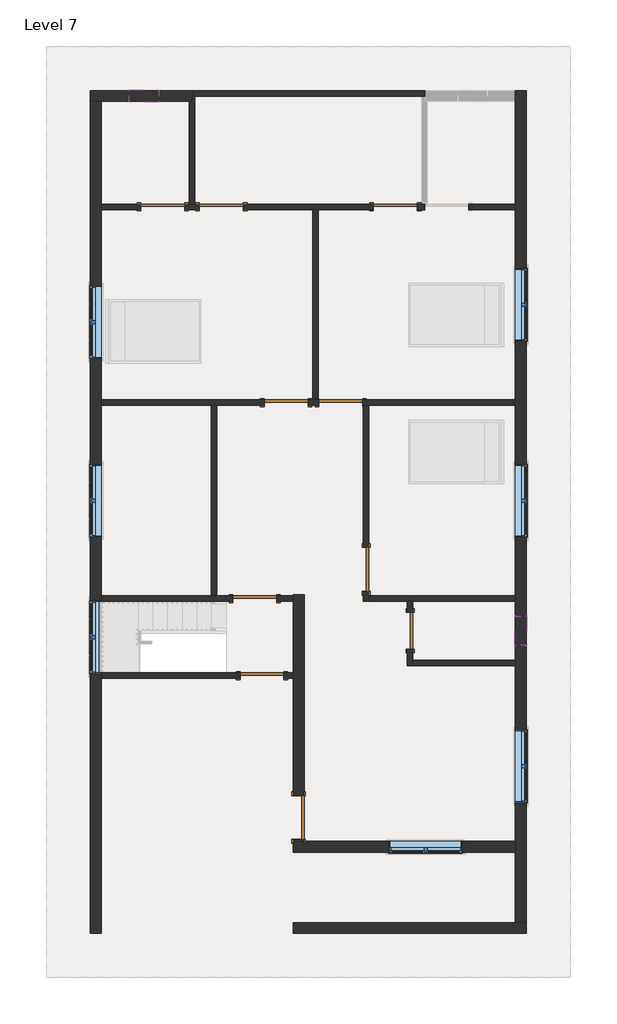
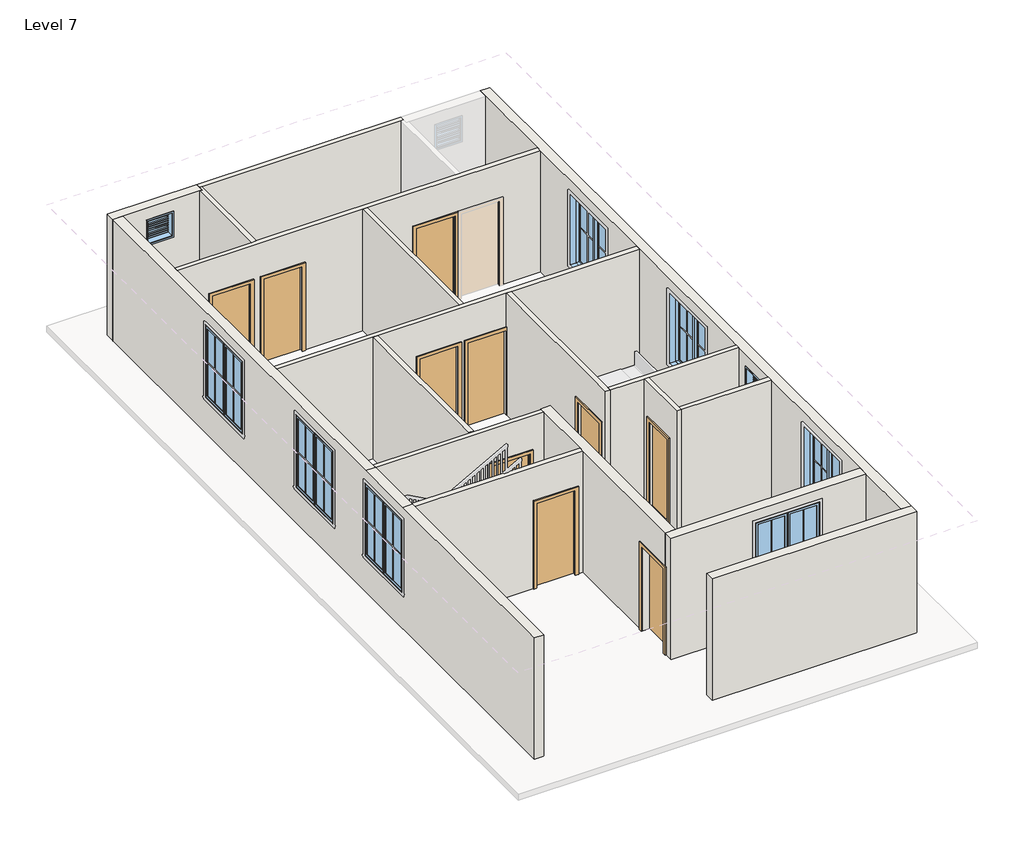
# One storey, part 1 of 3: 18 walls, 10 doors, 9 windows.
"""IFC4 building model written with IfcOpenShell, lengths in millimetres."""

from ifc_helpers import new_model, si_unit, frame, origin, place, context, project, spatial, polyline, outline, extrude, faceted_brep, transform, mapped, element, save
from components import door_78caadf7, single_flush_door_3_e5f9f3c4, single_flush_door_3_305aa2a5, single_flush_door_3_0ca8825f, window_casement_double_win_5_f93960c7, window_f2d8fef0

model = new_model("IFC4")

# Units and contexts
model_context = context("Model", 3, world=origin())
ifc_project = project(units=[si_unit("LENGTHUNIT", "METRE", prefix="MILLI")], contexts=[model_context])

# Site, building, storey
site = spatial("IfcSite", under=ifc_project)
building = spatial("IfcBuilding", under=site)
storey = spatial("IfcBuildingStorey", under=building, Name="Level 7", Elevation=16002.0)

# Doors
placement = place(None, origin())
door_shape = door_78caadf7(model_context)
element("IfcDoor", 1, ObjectType="Single-Flush : DOOR 2'6\"", at=placement, inside=storey, context=model_context, shape_type="MappedRepresentation", body=[
    mapped(door_shape, transform((860.2379845, -2779.6065691, 16002.0), x_axis=(0.0, 1.0, 0.0), y_axis=(-1.0, 0.0, 0.0), z_axis=(0.0, 0.0, 1.0))),
])
single_flush_door_3_shape = single_flush_door_3_e5f9f3c4(model_context)
element("IfcDoor", 2, ObjectType="Single-Flush : DOOR 3'", at=placement, inside=storey, context=model_context, shape_type="MappedRepresentation", body=[
    mapped(single_flush_door_3_shape, transform((-54.1620155, -1503.2565691, 16002.0), x_axis=(0.0, -1.0, 0.0), y_axis=(1.0, 0.0, 0.0), z_axis=(0.0, 0.0, 1.0))),
])
element("IfcDoor", 3, ObjectType="Single-Flush : DOOR 3'", at=placement, inside=storey, context=model_context, shape_type="MappedRepresentation", body=[
    mapped(single_flush_door_3_shape, transform((-1717.8620155, 1963.8434309, 16002.0), x_axis=(1.0, 0.0, 0.0), y_axis=(0.0, 1.0, 0.0), z_axis=(0.0, 0.0, 1.0))),
])
element("IfcDoor", 4, ObjectType="Single-Flush : DOOR 3'", at=placement, inside=storey, context=model_context, shape_type="MappedRepresentation", body=[
    mapped(single_flush_door_3_shape, transform((-2371.9120155, -2112.8565691, 16002.0), x_axis=(1.0, 0.0, 0.0), y_axis=(0.0, 1.0, 0.0), z_axis=(0.0, 0.0, 1.0))),
])
element("IfcDoor", 5, ObjectType="Single-Flush : DOOR 3'", at=placement, inside=storey, context=model_context, shape_type="MappedRepresentation", body=[
    mapped(single_flush_door_3_shape, transform((-2219.5120155, -3713.0565691, 16002.0), x_axis=(1.0, 0.0, 0.0), y_axis=(0.0, 1.0, 0.0), z_axis=(0.0, 0.0, 1.0))),
])
element("IfcDoor", 6, ObjectType="Single-Flush : DOOR 3'", at=placement, inside=storey, context=model_context, shape_type="MappedRepresentation", body=[
    mapped(single_flush_door_3_shape, transform((-4283.2620155, 6040.5434309, 16002.0), x_axis=(1.0, 0.0, 0.0), y_axis=(0.0, 1.0, 0.0), z_axis=(0.0, 0.0, 1.0))),
])
element("IfcDoor", 7, ObjectType="Single-Flush : DOOR 3'", at=placement, inside=storey, context=model_context, shape_type="MappedRepresentation", body=[
    mapped(single_flush_door_3_shape, transform((555.4379845, 6040.5434309, 16002.0), x_axis=(1.0, 0.0, 0.0), y_axis=(0.0, 1.0, 0.0), z_axis=(0.0, 0.0, 1.0))),
])
single_flush_door_3_2_shape = single_flush_door_3_305aa2a5(model_context)
element("IfcDoor", 8, ObjectType="Single-Flush : DOOR 3'", at=placement, inside=storey, context=model_context, shape_type="MappedRepresentation", body=[
    mapped(single_flush_door_3_2_shape, transform((-581.2120155, 1963.8434309, 16002.0), x_axis=(-1.0, 0.0, 0.0), y_axis=(0.0, -1.0, 0.0), z_axis=(0.0, 0.0, 1.0))),
])
element("IfcDoor", 9, ObjectType="Single-Flush : DOOR 3'", at=placement, inside=storey, context=model_context, shape_type="MappedRepresentation", body=[
    mapped(single_flush_door_3_2_shape, transform((-3064.0620155, 6040.5434309, 16002.0), x_axis=(-1.0, 0.0, 0.0), y_axis=(0.0, -1.0, 0.0), z_axis=(0.0, 0.0, 1.0))),
])
single_flush_door_3_3_shape = single_flush_door_3_0ca8825f(model_context)
element("IfcDoor", 10, ObjectType="Single-Flush : DOOR 3'", at=placement, inside=storey, context=model_context, shape_type="MappedRepresentation", body=[
    mapped(single_flush_door_3_3_shape, transform((-1457.5120155, -6665.8065691, 16002.0), x_axis=(0.0, -1.0, 0.0), y_axis=(1.0, 0.0, 0.0), z_axis=(0.0, 0.0, 1.0))),
])

# Walls
element("IfcWall", 11, ObjectType="WALL 4.5\"", at=placement, inside=storey, context=model_context, shape_type="Brep", body=[
    faceted_brep([(-3673.6620155, 8345.5934309, 16002.0), (-3616.5120155, 8345.5934309, 16002.0), (1107.8879845, 8345.5934309, 16002.0), (1165.0379845, 8345.5934309, 16002.0), (1165.0379845, 8345.5934309, 19050.0), (1107.8879845, 8345.5934309, 19050.0), (-3616.5120155, 8345.5934309, 19050.0), (-3673.6620155, 8345.5934309, 19050.0), (-3673.6620155, 8459.8934309, 16002.0), (-3673.6620155, 8459.8934309, 19050.0), (1165.0379845, 8459.8934309, 19050.0), (1165.0379845, 8459.8934309, 16002.0)], [[[0, 1, 2, 3, 4, 5, 6, 7]], [[8, 9, 10, 11]], [[3, 2, 1, 0, 8, 11]], [[4, 3, 11, 10]], [[0, 7, 9, 8]], [[7, 6, 5, 4, 10, 9]]]),
])
element("IfcWall", 12, ObjectType="WALL 4.5\"", at=placement, inside=storey, context=model_context, shape_type="SweptSolid", body=[
    extrude(outline(polyline([(-3730.8120155, 6097.6934309), (-3730.8120155, 8231.2934309), (-3673.6620155, 8231.2934309), (-3673.6620155, 8345.5934309), (-3616.5120155, 8345.5934309), (-3616.5120155, 6097.6934309), (-3730.8120155, 6097.6934309)])), frame((0.0, 0.0, 16002.0), z_axis=(0.0, 0.0, 1.0), x_axis=(1.0, 0.0, 0.0)), (0.0, 0.0, 1.0), 3048.0),
])
element("IfcWall", 13, ObjectType="WALL 4.5\"", at=placement, inside=storey, context=model_context, shape_type="Brep", body=[
    faceted_brep([(1165.0379845, 6097.6934309, 18135.6), (1165.0379845, 6097.6934309, 16002.0), (1107.8879845, 6097.6934309, 16002.0), (1012.6379845, 6097.6934309, 16002.0), (1012.6379845, 6097.6934309, 18135.6), (98.2379845, 6097.6934309, 18135.6), (98.2379845, 6097.6934309, 16002.0), (-2606.8620155, 6097.6934309, 16002.0), (-2606.8620155, 6097.6934309, 18135.6), (-3521.2620155, 6097.6934309, 18135.6), (-3521.2620155, 6097.6934309, 16002.0), (-3616.5120155, 6097.6934309, 16002.0), (-3730.8120155, 6097.6934309, 16002.0), (-3826.0620155, 6097.6934309, 16002.0), (-3826.0620155, 6097.6934309, 18135.6), (-4740.4620155, 6097.6934309, 18135.6), (-4740.4620155, 6097.6934309, 16002.0), (-5559.6120155, 6097.6934309, 16002.0), (-5559.6120155, 6097.6934309, 19050.0), (-3730.8120155, 6097.6934309, 19050.0), (-3616.5120155, 6097.6934309, 19050.0), (1107.8879845, 6097.6934309, 19050.0), (1222.1879845, 6097.6934309, 19050.0), (3050.9879845, 6097.6934309, 19050.0), (3050.9879845, 6097.6934309, 16002.0), (2079.4379845, 6097.6934309, 16002.0), (2079.4379845, 6097.6934309, 18135.6), (1012.6379845, 5983.3934309, 16002.0), (1165.0379845, 5983.3934309, 16002.0), (1165.0379845, 5983.3934309, 18135.6), (2079.4379845, 5983.3934309, 18135.6), (2079.4379845, 5983.3934309, 16002.0), (3050.9879845, 5983.3934309, 16002.0), (3050.9879845, 5983.3934309, 19050.0), (-1051.1120155, 5983.3934309, 19050.0), (-1165.4120155, 5983.3934309, 19050.0), (-5559.6120155, 5983.3934309, 19050.0), (-5559.6120155, 5983.3934309, 16002.0), (-4740.4620155, 5983.3934309, 16002.0), (-4740.4620155, 5983.3934309, 18135.6), (-3826.0620155, 5983.3934309, 18135.6), (-3826.0620155, 5983.3934309, 16002.0), (-3521.2620155, 5983.3934309, 16002.0), (-3521.2620155, 5983.3934309, 18135.6), (-2606.8620155, 5983.3934309, 18135.6), (-2606.8620155, 5983.3934309, 16002.0), (-1165.4120155, 5983.3934309, 16002.0), (-1051.1120155, 5983.3934309, 16002.0), (98.2379845, 5983.3934309, 16002.0), (98.2379845, 5983.3934309, 18135.6), (1012.6379845, 5983.3934309, 18135.6)], [[[0, 1, 2, 3, 4, 5, 6, 7, 8, 9, 10, 11, 12, 13, 14, 15, 16, 17, 18, 19, 20, 21, 22, 23, 24, 25, 26]], [[27, 28, 29, 30, 31, 32, 33, 34, 35, 36, 37, 38, 39, 40, 41, 42, 43, 44, 45, 46, 47, 48, 49, 50]], [[38, 37, 17, 16]], [[13, 12, 11, 10, 42, 41]], [[48, 47, 46, 45, 7, 6]], [[25, 24, 32, 31]], [[3, 2, 1, 28, 27]], [[18, 17, 37, 36]], [[24, 23, 33, 32]], [[14, 13, 41, 40]], [[15, 14, 40, 39]], [[16, 15, 39, 38]], [[43, 42, 10, 9]], [[44, 43, 9, 8]], [[45, 44, 8, 7]], [[4, 3, 27, 50]], [[5, 4, 50, 49]], [[6, 5, 49, 48]], [[29, 28, 1, 0]], [[30, 29, 0, 26]], [[31, 30, 26, 25]], [[23, 22, 21, 20, 19, 18, 36, 35, 34, 33]]]),
])
element("IfcWall", 14, ObjectType="WALL 4.5\"", at=placement, inside=storey, context=model_context, shape_type="SweptSolid", body=[
    extrude(outline(polyline([(-1165.4120155, 2020.9934309), (-1165.4120155, 5983.3934309), (-1051.1120155, 5983.3934309), (-1051.1120155, 2020.9934309), (-1165.4120155, 2020.9934309)])), frame((0.0, 0.0, 16002.0), z_axis=(0.0, 0.0, 1.0), x_axis=(1.0, 0.0, 0.0)), (0.0, 0.0, 1.0), 3048.0),
])
element("IfcWall", 15, ObjectType="WALL 4.5\"", at=placement, inside=storey, context=model_context, shape_type="Brep", body=[
    faceted_brep([(-1260.6620155, 1906.6934309, 18135.6), (-1260.6620155, 1906.6934309, 16002.0), (-1038.4120155, 1906.6934309, 16002.0), (-1038.4120155, 1906.6934309, 18135.6), (-124.0120155, 1906.6934309, 18135.6), (-124.0120155, 1906.6934309, 16002.0), (-111.3120155, 1906.6934309, 16002.0), (2.9879845, 1906.6934309, 16002.0), (3050.9879845, 1906.6934309, 16002.0), (3050.9879845, 1906.6934309, 19050.0), (2.9879845, 1906.6934309, 19050.0), (-111.3120155, 1906.6934309, 19050.0), (-3159.3120155, 1906.6934309, 19050.0), (-3273.6120155, 1906.6934309, 19050.0), (-5559.6120155, 1906.6934309, 19050.0), (-5559.6120155, 1906.6934309, 16002.0), (-3273.6120155, 1906.6934309, 16002.0), (-3159.3120155, 1906.6934309, 16002.0), (-2175.0620155, 1906.6934309, 16002.0), (-2175.0620155, 1906.6934309, 18135.6), (-1038.4120155, 2020.9934309, 16002.0), (-1051.1120155, 2020.9934309, 16002.0), (-1165.4120155, 2020.9934309, 16002.0), (-1260.6620155, 2020.9934309, 16002.0), (-1260.6620155, 2020.9934309, 18135.6), (-2175.0620155, 2020.9934309, 18135.6), (-2175.0620155, 2020.9934309, 16002.0), (-5559.6120155, 2020.9934309, 16002.0), (-5559.6120155, 2020.9934309, 19050.0), (-1165.4120155, 2020.9934309, 19050.0), (-1051.1120155, 2020.9934309, 19050.0), (3050.9879845, 2020.9934309, 19050.0), (3050.9879845, 2020.9934309, 16002.0), (-124.0120155, 2020.9934309, 16002.0), (-124.0120155, 2020.9934309, 18135.6), (-1038.4120155, 2020.9934309, 18135.6)], [[[0, 1, 2, 3, 4, 5, 6, 7, 8, 9, 10, 11, 12, 13, 14, 15, 16, 17, 18, 19]], [[20, 21, 22, 23, 24, 25, 26, 27, 28, 29, 30, 31, 32, 33, 34, 35]], [[33, 32, 8, 7, 6, 5]], [[2, 1, 23, 22, 21, 20]], [[18, 17, 16, 15, 27, 26]], [[15, 14, 28, 27]], [[9, 8, 32, 31]], [[3, 2, 20, 35]], [[4, 3, 35, 34]], [[5, 4, 34, 33]], [[24, 23, 1, 0]], [[25, 24, 0, 19]], [[26, 25, 19, 18]], [[14, 13, 12, 11, 10, 9, 31, 30, 29, 28]]]),
])
element("IfcWall", 16, ObjectType="WALL 4.5\"", at=placement, inside=storey, context=model_context, shape_type="SweptSolid", body=[
    extrude(outline(polyline([(-3273.6120155, -2032.8465691), (-3273.6120155, 1906.6934309), (-3159.3120155, 1906.6934309), (-3159.3120155, -2032.8465691), (-3273.6120155, -2032.8465691)])), frame((0.0, 0.0, 16002.0), z_axis=(0.0, 0.0, 1.0), x_axis=(1.0, 0.0, 0.0)), (0.0, 0.0, 1.0), 3048.0),
])
element("IfcWall", 17, ObjectType="WALL 4.5\"", at=placement, inside=storey, context=model_context, shape_type="SweptSolid", body=[
    extrude(outline(polyline([(18135.6, -1914.7120155), (16002.0, -1914.7120155), (16002.0, -1571.8120155), (19050.0, -1571.8120155), (19050.0, -5559.6120155), (16002.0, -5559.6120155), (16002.0, -2829.1120155), (18135.6, -2829.1120155), (18135.6, -1914.7120155)])), frame((0.0, -2170.0065691, 0.0), z_axis=(0.0, 1.0, 0.0), x_axis=(0.0, 0.0, 1.0)), (0.0, 0.0, 1.0), 114.3),
])
element("IfcWall", 18, ObjectType="WALL 4.5\"", at=placement, inside=storey, context=model_context, shape_type="SweptSolid", body=[
    extrude(outline(polyline([(18135.6, -1762.3120155), (16002.0, -1762.3120155), (16002.0, -1571.8120155), (19050.0, -1571.8120155), (19050.0, -5559.6120155), (16002.0, -5559.6120155), (16002.0, -2676.7120155), (18135.6, -2676.7120155), (18135.6, -1762.3120155)])), frame((0.0, -3770.2065691, 0.0), z_axis=(0.0, 1.0, 0.0), x_axis=(0.0, 0.0, 1.0)), (0.0, 0.0, 1.0), 114.3),
])
element("IfcWall", 19, ObjectType="WALL 4.5\"", at=placement, inside=storey, context=model_context, shape_type="Brep", body=[
    faceted_brep([(-111.3120155, -1960.4565691, 18135.6), (-111.3120155, -1960.4565691, 16002.0), (-111.3120155, -2170.0065691, 16002.0), (-111.3120155, -2170.0065691, 19050.0), (-111.3120155, 1906.6934309, 19050.0), (-111.3120155, 1906.6934309, 16002.0), (-111.3120155, -1046.0565691, 16002.0), (-111.3120155, -1046.0565691, 18135.6), (2.9879845, -2170.0065691, 16002.0), (2.9879845, -2055.7065691, 16002.0), (2.9879845, -1960.4565691, 16002.0), (2.9879845, -1960.4565691, 18135.6), (2.9879845, -1046.0565691, 18135.6), (2.9879845, -1046.0565691, 16002.0), (2.9879845, 1906.6934309, 16002.0), (2.9879845, 1906.6934309, 19050.0), (2.9879845, -2055.7065691, 19050.0), (2.9879845, -2170.0065691, 19050.0)], [[[0, 1, 2, 3, 4, 5, 6, 7]], [[8, 9, 10, 11, 12, 13, 14, 15, 16, 17]], [[6, 5, 14, 13]], [[2, 1, 10, 9, 8]], [[5, 4, 15, 14]], [[3, 2, 8, 17]], [[11, 10, 1, 0]], [[12, 11, 0, 7]], [[13, 12, 7, 6]], [[4, 3, 17, 16, 15]]]),
])
element("IfcWall", 20, ObjectType="WALL 4.5\"", at=placement, inside=storey, context=model_context, shape_type="Brep", body=[
    faceted_brep([(2.9879845, -2170.0065691, 16002.0), (803.0879845, -2170.0065691, 16002.0), (917.3879845, -2170.0065691, 16002.0), (3050.9879845, -2170.0065691, 16002.0), (3050.9879845, -2170.0065691, 19050.0), (917.3879845, -2170.0065691, 19050.0), (803.0879845, -2170.0065691, 19050.0), (2.9879845, -2170.0065691, 19050.0), (2.9879845, -2055.7065691, 16002.0), (2.9879845, -2055.7065691, 19050.0), (3050.9879845, -2055.7065691, 19050.0), (3050.9879845, -2055.7065691, 16002.0)], [[[0, 1, 2, 3, 4, 5, 6, 7]], [[8, 9, 10, 11]], [[3, 2, 1, 0, 8, 11]], [[0, 7, 9, 8]], [[4, 3, 11, 10]], [[7, 6, 5, 4, 10, 9]]]),
])
element("IfcWall", 21, ObjectType="WALL 4.5\"", at=placement, inside=storey, context=model_context, shape_type="Brep", body=[
    faceted_brep([(803.0879845, -2170.0065691, 16002.0), (803.0879845, -2398.6065691, 16002.0), (803.0879845, -2398.6065691, 18135.6), (803.0879845, -3160.6065691, 18135.6), (803.0879845, -3160.6065691, 16002.0), (803.0879845, -3503.5065691, 16002.0), (803.0879845, -3503.5065691, 19050.0), (803.0879845, -2170.0065691, 19050.0), (917.3879845, -2398.6065691, 18135.6), (917.3879845, -2398.6065691, 16002.0), (917.3879845, -2170.0065691, 16002.0), (917.3879845, -2170.0065691, 19050.0), (917.3879845, -3389.2065691, 19050.0), (917.3879845, -3503.5065691, 19050.0), (917.3879845, -3503.5065691, 16002.0), (917.3879845, -3389.2065691, 16002.0), (917.3879845, -3160.6065691, 16002.0), (917.3879845, -3160.6065691, 18135.6)], [[[0, 1, 2, 3, 4, 5, 6, 7]], [[8, 9, 10, 11, 12, 13, 14, 15, 16, 17]], [[10, 9, 1, 0]], [[16, 15, 14, 5, 4]], [[0, 7, 11, 10]], [[6, 5, 14, 13]], [[2, 1, 9, 8]], [[3, 2, 8, 17]], [[4, 3, 17, 16]], [[7, 6, 13, 12, 11]]]),
])
element("IfcWall", 22, ObjectType="WALL 4.5\"", at=placement, inside=storey, context=model_context, shape_type="SweptSolid", body=[
    extrude(outline(polyline([(917.3879845, -3389.2065691), (3050.9879845, -3389.2065691), (3050.9879845, -3503.5065691), (917.3879845, -3503.5065691), (917.3879845, -3389.2065691)])), frame((0.0, 0.0, 16002.0), z_axis=(0.0, 0.0, 1.0), x_axis=(1.0, 0.0, 0.0)), (0.0, 0.0, 1.0), 3048.0),
])
element("IfcWall", 23, ObjectType="WALL 9\"", at=placement, inside=storey, context=model_context, shape_type="Brep", body=[
    faceted_brep([(-3673.6620155, 8459.8934309, 16002.0), (-5788.2120155, 8459.8934309, 16002.0), (-5788.2120155, 8459.8934309, 19050.0), (-3673.6620155, 8459.8934309, 19050.0), (-4978.5870155, 8459.8934309, 18745.2), (-4978.5870155, 8459.8934309, 18135.6), (-4368.9870155, 8459.8934309, 18135.6), (-4368.9870155, 8459.8934309, 18745.2), (-3673.6620155, 8231.2934309, 16002.0), (-3673.6620155, 8231.2934309, 19050.0), (-3730.8120155, 8231.2934309, 19050.0), (-5559.6120155, 8231.2934309, 19050.0), (-5788.2120155, 8231.2934309, 19050.0), (-5788.2120155, 8231.2934309, 16002.0), (-5559.6120155, 8231.2934309, 16002.0), (-3730.8120155, 8231.2934309, 16002.0), (-4978.5870155, 8231.2934309, 18745.2), (-4368.9870155, 8231.2934309, 18745.2), (-4368.9870155, 8231.2934309, 18135.6), (-4978.5870155, 8231.2934309, 18135.6), (-3673.6620155, 8345.5934309, 16002.0), (-3673.6620155, 8345.5934309, 19050.0)], [[[0, 1, 2, 3], [4, 5, 6, 7]], [[8, 9, 10, 11, 12, 13, 14, 15], [16, 17, 18, 19]], [[1, 0, 20, 8, 15, 14, 13]], [[0, 3, 21, 9, 8, 20]], [[2, 1, 13, 12]], [[5, 4, 16, 19]], [[6, 5, 19, 18]], [[7, 6, 18, 17]], [[4, 7, 17, 16]], [[3, 2, 12, 11, 10, 9, 21]]]),
])
element("IfcWall", 24, ObjectType="WALL 9\"", at=placement, inside=storey, context=model_context, shape_type="Brep", body=[
    faceted_brep([(-5788.2120155, 8231.2934309, 16002.0), (-5788.2120155, -9078.8065691, 16002.0), (-5788.2120155, -9078.8065691, 19050.0), (-5788.2120155, -3674.9565691, 19050.0), (-5788.2120155, -2150.9565691, 19050.0), (-5788.2120155, 8231.2934309, 19050.0), (-5788.2120155, 4402.2434309, 18745.2), (-5788.2120155, 2878.2434309, 18745.2), (-5788.2120155, 2878.2434309, 16916.4), (-5788.2120155, 4402.2434309, 16916.4), (-5788.2120155, -2150.9565691, 18745.2), (-5788.2120155, -3674.9565691, 18745.2), (-5788.2120155, -3674.9565691, 16916.4), (-5788.2120155, -2150.9565691, 16916.4), (-5788.2120155, 687.4934309, 18745.2), (-5788.2120155, -836.5065691, 18745.2), (-5788.2120155, -836.5065691, 16916.4), (-5788.2120155, 687.4934309, 16916.4), (-5559.6120155, 8231.2934309, 16002.0), (-5559.6120155, 8231.2934309, 19050.0), (-5559.6120155, 6097.6934309, 19050.0), (-5559.6120155, 5983.3934309, 19050.0), (-5559.6120155, 2020.9934309, 19050.0), (-5559.6120155, 1906.6934309, 19050.0), (-5559.6120155, -2055.7065691, 19050.0), (-5559.6120155, -2150.9565691, 19050.0), (-5559.6120155, -2170.0065691, 19050.0), (-5559.6120155, -3655.9065691, 19050.0), (-5559.6120155, -3674.9565691, 19050.0), (-5559.6120155, -3770.2065691, 19050.0), (-5559.6120155, -9078.8065691, 19050.0), (-5559.6120155, -9078.8065691, 16002.0), (-5559.6120155, -3770.2065691, 16002.0), (-5559.6120155, -3655.9065691, 16002.0), (-5559.6120155, -2170.0065691, 16002.0), (-5559.6120155, -2055.7065691, 16002.0), (-5559.6120155, 1906.6934309, 16002.0), (-5559.6120155, 2020.9934309, 16002.0), (-5559.6120155, 5983.3934309, 16002.0), (-5559.6120155, 6097.6934309, 16002.0), (-5559.6120155, 4402.2434309, 18745.2), (-5559.6120155, 4402.2434309, 16916.4), (-5559.6120155, 2878.2434309, 16916.4), (-5559.6120155, 2878.2434309, 18745.2), (-5559.6120155, -2150.9565691, 18745.2), (-5559.6120155, -2150.9565691, 16916.4), (-5559.6120155, -3674.9565691, 16916.4), (-5559.6120155, -3674.9565691, 18745.2), (-5559.6120155, 687.4934309, 18745.2), (-5559.6120155, 687.4934309, 16916.4), (-5559.6120155, -836.5065691, 16916.4), (-5559.6120155, -836.5065691, 18745.2)], [[[0, 1, 2, 3, 4, 5], [6, 7, 8, 9], [10, 11, 12, 13], [14, 15, 16, 17]], [[18, 19, 20, 21, 22, 23, 24, 25, 26, 27, 28, 29, 30, 31, 32, 33, 34, 35, 36, 37, 38, 39], [40, 41, 42, 43], [44, 45, 46, 47], [48, 49, 50, 51]], [[1, 0, 18, 39, 38, 37, 36, 35, 34, 33, 32, 31]], [[2, 1, 31, 30]], [[0, 5, 19, 18]], [[41, 40, 6, 9]], [[42, 41, 9, 8]], [[43, 42, 8, 7]], [[40, 43, 7, 6]], [[45, 44, 10, 13]], [[46, 45, 13, 12]], [[47, 46, 12, 11]], [[44, 47, 11, 10]], [[49, 48, 14, 17]], [[50, 49, 17, 16]], [[51, 50, 16, 15]], [[48, 51, 15, 14]], [[4, 3, 28, 27, 26, 25]], [[3, 2, 30, 29, 28]], [[5, 4, 25, 24, 23, 22, 21, 20, 19]]]),
])
element("IfcWall", 25, ObjectType="WALL 9\"", at=placement, inside=storey, context=model_context, shape_type="Brep", body=[
    faceted_brep([(-1571.8120155, -9078.8065691, 16002.0), (3279.5879845, -9078.8065691, 16002.0), (3279.5879845, -9078.8065691, 19050.0), (-1571.8120155, -9078.8065691, 19050.0), (-1571.8120155, -8850.2065691, 16002.0), (-1571.8120155, -8850.2065691, 19050.0), (3050.9879845, -8850.2065691, 19050.0), (3279.5879845, -8850.2065691, 19050.0), (3279.5879845, -8850.2065691, 16002.0), (3050.9879845, -8850.2065691, 16002.0)], [[[0, 1, 2, 3]], [[4, 5, 6, 7, 8, 9]], [[1, 0, 4, 9, 8]], [[0, 3, 5, 4]], [[2, 1, 8, 7]], [[3, 2, 7, 6, 5]]]),
])
element("IfcWall", 26, ObjectType="WALL 9\"", at=placement, inside=storey, context=model_context, shape_type="Brep", body=[
    faceted_brep([(3279.5879845, -8850.2065691, 16002.0), (3279.5879845, 8459.8934309, 16002.0), (3279.5879845, 8459.8934309, 19050.0), (3279.5879845, -8850.2065691, 19050.0), (3279.5879845, 3240.1934309, 18745.2), (3279.5879845, 4764.1934309, 18745.2), (3279.5879845, 4764.1934309, 16916.4), (3279.5879845, 3240.1934309, 16916.4), (3279.5879845, -836.5065691, 18745.2), (3279.5879845, 687.4934309, 18745.2), (3279.5879845, 687.4934309, 16916.4), (3279.5879845, -836.5065691, 16916.4), (3279.5879845, -6361.0065691, 18745.2), (3279.5879845, -4837.0065691, 18745.2), (3279.5879845, -4837.0065691, 16916.4), (3279.5879845, -6361.0065691, 16916.4), (3279.5879845, -2474.8065691, 18745.2), (3279.5879845, -2474.8065691, 18135.6), (3279.5879845, -3084.4065691, 18135.6), (3279.5879845, -3084.4065691, 18745.2), (3050.9879845, -8850.2065691, 16002.0), (3050.9879845, -8850.2065691, 19050.0), (3050.9879845, -7389.7065691, 19050.0), (3050.9879845, -7161.1065691, 19050.0), (3050.9879845, -3503.5065691, 19050.0), (3050.9879845, -3389.2065691, 19050.0), (3050.9879845, -2170.0065691, 19050.0), (3050.9879845, -2055.7065691, 19050.0), (3050.9879845, 1906.6934309, 19050.0), (3050.9879845, 2020.9934309, 19050.0), (3050.9879845, 5983.3934309, 19050.0), (3050.9879845, 6097.6934309, 19050.0), (3050.9879845, 8231.2934309, 19050.0), (3050.9879845, 8459.8934309, 19050.0), (3050.9879845, 8459.8934309, 16002.0), (3050.9879845, 8231.2934309, 16002.0), (3050.9879845, 6097.6934309, 16002.0), (3050.9879845, 5983.3934309, 16002.0), (3050.9879845, 2020.9934309, 16002.0), (3050.9879845, 1906.6934309, 16002.0), (3050.9879845, -2055.7065691, 16002.0), (3050.9879845, -2170.0065691, 16002.0), (3050.9879845, -3389.2065691, 16002.0), (3050.9879845, -3503.5065691, 16002.0), (3050.9879845, -7161.1065691, 16002.0), (3050.9879845, -7389.7065691, 16002.0), (3050.9879845, 3240.1934309, 18745.2), (3050.9879845, 3240.1934309, 16916.4), (3050.9879845, 4764.1934309, 16916.4), (3050.9879845, 4764.1934309, 18745.2), (3050.9879845, -836.5065691, 18745.2), (3050.9879845, -836.5065691, 16916.4), (3050.9879845, 687.4934309, 16916.4), (3050.9879845, 687.4934309, 18745.2), (3050.9879845, -6361.0065691, 18745.2), (3050.9879845, -6361.0065691, 16916.4), (3050.9879845, -4837.0065691, 16916.4), (3050.9879845, -4837.0065691, 18745.2), (3050.9879845, -2474.8065691, 18745.2), (3050.9879845, -3084.4065691, 18745.2), (3050.9879845, -3084.4065691, 18135.6), (3050.9879845, -2474.8065691, 18135.6)], [[[0, 1, 2, 3], [4, 5, 6, 7], [8, 9, 10, 11], [12, 13, 14, 15], [16, 17, 18, 19]], [[20, 21, 22, 23, 24, 25, 26, 27, 28, 29, 30, 31, 32, 33, 34, 35, 36, 37, 38, 39, 40, 41, 42, 43, 44, 45], [46, 47, 48, 49], [50, 51, 52, 53], [54, 55, 56, 57], [58, 59, 60, 61]], [[1, 0, 20, 45, 44, 43, 42, 41, 40, 39, 38, 37, 36, 35, 34]], [[0, 3, 21, 20]], [[2, 1, 34, 33]], [[47, 46, 4, 7]], [[48, 47, 7, 6]], [[49, 48, 6, 5]], [[46, 49, 5, 4]], [[51, 50, 8, 11]], [[52, 51, 11, 10]], [[53, 52, 10, 9]], [[50, 53, 9, 8]], [[55, 54, 12, 15]], [[56, 55, 15, 14]], [[57, 56, 14, 13]], [[54, 57, 13, 12]], [[17, 16, 58, 61]], [[18, 17, 61, 60]], [[19, 18, 60, 59]], [[16, 19, 59, 58]], [[3, 2, 33, 32, 31, 30, 29, 28, 27, 26, 25, 24, 23, 22, 21]]]),
])
element("IfcWall", 27, ObjectType="WALL 9\"", at=placement, inside=storey, context=model_context, shape_type="Brep", body=[
    faceted_brep([(3050.9879845, -7161.1065691, 16002.0), (-1343.2120155, -7161.1065691, 16002.0), (-1571.8120155, -7161.1065691, 16002.0), (-1571.8120155, -7161.1065691, 19050.0), (-1343.2120155, -7161.1065691, 19050.0), (3050.9879845, -7161.1065691, 19050.0), (422.0879845, -7161.1065691, 18745.2), (422.0879845, -7161.1065691, 16916.4), (1946.0879845, -7161.1065691, 16916.4), (1946.0879845, -7161.1065691, 18745.2), (3050.9879845, -7389.7065691, 16002.0), (3050.9879845, -7389.7065691, 19050.0), (-1571.8120155, -7389.7065691, 19050.0), (-1571.8120155, -7389.7065691, 16002.0), (422.0879845, -7389.7065691, 18745.2), (1946.0879845, -7389.7065691, 18745.2), (1946.0879845, -7389.7065691, 16916.4), (422.0879845, -7389.7065691, 16916.4)], [[[0, 1, 2, 3, 4, 5], [6, 7, 8, 9]], [[10, 11, 12, 13], [14, 15, 16, 17]], [[2, 1, 0, 10, 13]], [[0, 5, 11, 10]], [[3, 2, 13, 12]], [[7, 6, 14, 17]], [[8, 7, 17, 16]], [[9, 8, 16, 15]], [[6, 9, 15, 14]], [[5, 4, 3, 12, 11]]]),
])
element("IfcWall", 28, ObjectType="WALL 9\"", at=placement, inside=storey, context=model_context, shape_type="Brep", body=[
    faceted_brep([(-1343.2120155, -7161.1065691, 16002.0), (-1343.2120155, -7123.0065691, 16002.0), (-1343.2120155, -7123.0065691, 18135.6), (-1343.2120155, -6208.6065691, 18135.6), (-1343.2120155, -6208.6065691, 16002.0), (-1343.2120155, -2032.8465691, 16002.0), (-1343.2120155, -2032.8465691, 19050.0), (-1343.2120155, -7161.1065691, 19050.0), (-1571.8120155, -7123.0065691, 18135.6), (-1571.8120155, -7123.0065691, 16002.0), (-1571.8120155, -7161.1065691, 16002.0), (-1571.8120155, -7161.1065691, 19050.0), (-1571.8120155, -3770.2065691, 19050.0), (-1571.8120155, -3655.9065691, 19050.0), (-1571.8120155, -2170.0065691, 19050.0), (-1571.8120155, -2055.7065691, 19050.0), (-1571.8120155, -2032.8465691, 19050.0), (-1571.8120155, -2032.8465691, 16002.0), (-1571.8120155, -2055.7065691, 16002.0), (-1571.8120155, -2170.0065691, 16002.0), (-1571.8120155, -3655.9065691, 16002.0), (-1571.8120155, -3770.2065691, 16002.0), (-1571.8120155, -6208.6065691, 16002.0), (-1571.8120155, -6208.6065691, 18135.6)], [[[0, 1, 2, 3, 4, 5, 6, 7]], [[8, 9, 10, 11, 12, 13, 14, 15, 16, 17, 18, 19, 20, 21, 22, 23]], [[10, 9, 1, 0]], [[22, 21, 20, 19, 18, 17, 5, 4]], [[6, 5, 17, 16]], [[0, 7, 11, 10]], [[2, 1, 9, 8]], [[3, 2, 8, 23]], [[4, 3, 23, 22]], [[7, 6, 16, 15, 14, 13, 12, 11]]]),
])

# Windows
window_casement_double_win_5_shape = window_casement_double_win_5_f93960c7(model_context)
element("IfcWindow", 29, ObjectType="Window-Casement-Double : WIN 5'", at=placement, inside=storey, context=model_context, shape_type="MappedRepresentation", body=[
    mapped(window_casement_double_win_5_shape, transform((-5673.9120155, 3640.2434309, 16002.0), x_axis=(0.0, 1.0, 0.0), y_axis=(-1.0, 0.0, 0.0), z_axis=(0.0, 0.0, 1.0))),
])
element("IfcWindow", 30, ObjectType="Window-Casement-Double : WIN 5'", at=placement, inside=storey, context=model_context, shape_type="MappedRepresentation", body=[
    mapped(window_casement_double_win_5_shape, transform((3165.2879845, 4002.1934309, 16002.0), x_axis=(0.0, -1.0, 0.0), y_axis=(1.0, 0.0, 0.0), z_axis=(0.0, 0.0, 1.0))),
])
element("IfcWindow", 31, ObjectType="Window-Casement-Double : WIN 5'", at=placement, inside=storey, context=model_context, shape_type="MappedRepresentation", body=[
    mapped(window_casement_double_win_5_shape, transform((3165.2879845, -74.5065691, 16002.0), x_axis=(0.0, -1.0, 0.0), y_axis=(1.0, 0.0, 0.0), z_axis=(0.0, 0.0, 1.0))),
])
element("IfcWindow", 32, ObjectType="Window-Casement-Double : WIN 5'", at=placement, inside=storey, context=model_context, shape_type="MappedRepresentation", body=[
    mapped(window_casement_double_win_5_shape, transform((3165.2879845, -5599.0065691, 16002.0), x_axis=(0.0, -1.0, 0.0), y_axis=(1.0, 0.0, 0.0), z_axis=(0.0, 0.0, 1.0))),
])
element("IfcWindow", 33, ObjectType="Window-Casement-Double : WIN 5'", at=placement, inside=storey, context=model_context, shape_type="MappedRepresentation", body=[
    mapped(window_casement_double_win_5_shape, transform((1184.0879845, -7275.4065691, 16002.0), x_axis=(-1.0, 0.0, 0.0), y_axis=(0.0, -1.0, 0.0), z_axis=(0.0, 0.0, 1.0))),
])
element("IfcWindow", 34, ObjectType="Window-Casement-Double : WIN 5'", at=placement, inside=storey, context=model_context, shape_type="MappedRepresentation", body=[
    mapped(window_casement_double_win_5_shape, transform((-5673.9120155, -2912.9565691, 16002.0), x_axis=(0.0, 1.0, 0.0), y_axis=(-1.0, 0.0, 0.0), z_axis=(0.0, 0.0, 1.0))),
])
element("IfcWindow", 35, ObjectType="Window-Casement-Double : WIN 5'", at=placement, inside=storey, context=model_context, shape_type="MappedRepresentation", body=[
    mapped(window_casement_double_win_5_shape, transform((-5673.9120155, -74.5065691, 16002.0), x_axis=(0.0, 1.0, 0.0), y_axis=(-1.0, 0.0, 0.0), z_axis=(0.0, 0.0, 1.0))),
])
window_shape = window_f2d8fef0(model_context)
element("IfcWindow", 36, ObjectType="Window-Louvers : 24\" x 24\"", at=placement, inside=storey, context=model_context, shape_type="MappedRepresentation", body=[
    mapped(window_shape, transform((-4673.7870155, 8351.9434309, 17221.2), x_axis=(1.0, 0.0, 0.0), y_axis=(0.0, 1.0, 0.0), z_axis=(0.0, 0.0, 1.0))),
])
element("IfcWindow", 37, ObjectType="Window-Louvers : 24\" x 24\"", at=placement, inside=storey, context=model_context, shape_type="MappedRepresentation", body=[
    mapped(window_shape, transform((3171.6379845, -2779.6065691, 17221.2), x_axis=(0.0, -1.0, 0.0), y_axis=(1.0, 0.0, 0.0), z_axis=(0.0, 0.0, 1.0))),
])

save(model, "model.ifc")

# Revit data of these elements
# Type "Single-Flush : DOOR 2'6\""
#   Type Mark = "10"
#   Construction Type Id = "MDOOR"
#   Assembly Code = "C1020"
#   Analytic Construction = "Metal"
#   Thickness = 0' - 2"
#   Heat Transfer Coefficient (U) = 0.651978 BTU/(h·ft²·°F)
#   Height = 7' - 0"
#   Trim Projection Ext = 0' - 1"
#   Trim Projection Int = 0' - 1"
#   Trim Width = 0' - 3"
#   Width = 2' - 6"
#   Define Thermal Properties by = 1
#   Door Material = Door - Panel
#   Frame Material = Door - Frame
#   Visual Light Transmittance = 0
#   Solar Heat Gain Coefficient = 0
#   Function = (empty or 0)
#   Wall Closure = (empty or 0)
# Type "Single-Flush : DOOR 3'"
#   Type Mark = "9"
#   Construction Type Id = "MDOOR"
#   Assembly Code = "C1020"
#   Analytic Construction = "Metal"
#   Thickness = 0' - 2"
#   Heat Transfer Coefficient (U) = 0.651978 BTU/(h·ft²·°F)
#   Height = 7' - 0"
#   Trim Projection Ext = 0' - 1"
#   Trim Projection Int = 0' - 1"
#   Trim Width = 0' - 3"
#   Width = 3' - 0"
#   Define Thermal Properties by = 1
#   Door Material = Door - Panel
#   Frame Material = Door - Frame
#   Visual Light Transmittance = 0
#   Solar Heat Gain Coefficient = 0
#   Function = (empty or 0)
#   Wall Closure = (empty or 0)
# Type "WALL 4.5\""
#   Assembly Code = "B2010"
#   Layers, outside or top first: 0' - 4 1/2" no material (function 1)
# Type "WALL 9\""
#   Assembly Code = "B2010"
#   Layers, outside or top first: 0' - 9" no material (function 1)
# Type "Window-Casement-Double : WIN 5'"
#   Type Mark = "18"
#   Fire Rating = "0.5h"
#   Assembly Code = "B2020100"
#   Analytic Construction = "Double glazing - domestic"
#   Frame Extension [instance default] = 0' - 0 1/4"
#   Window Inset [instance default] = 0' - 0"
#   Wall Thickness [instance default] = 0' - 6"
#   Interior Wall Closure [instance default] = 0' - 2 1/4"
#   Half Width = 2' - 6"
#   Visual Light Transmittance = 0.81
#   Thermal Resistance (R) = 1.8146 (h·ft²·°F)/BTU
#   Solar Heat Gain Coefficient = 0.76
#   Rough Width = 5' - 0 1/2"
#   Rough Height = 6' - 0 1/2"
#   Height = 6' - 0"
#   Heat Transfer Coefficient (U) = 0.5511 BTU/(h·ft²·°F)
#   Exterior Wall Closure [instance default] = 0' - 1 1/4"
#   Extension Jamb [instance default] = 0' - 2 1/4"
#   Default Sill Height = 3' - 0"
#   Width = 5' - 0"
#   Muntin Visibility = yes
#   Interior Trim Visibility [instance default] = yes
#   Exterior Trim Visibility [instance default] = yes
#   Extension Jamb Visibility [instance default] = yes
#   Interior Trim Material = Wood - Stained
#   Muntin Pattern = Muntin Pattern_2x2 : Muntin Pattern_2x2
#   Interior Trim = Trim-Window-Interior-Flat : Picture Frame
#   Interior Frame Material = Wood - Stained
#   Glass Panel Material = Glass
#   Exterior Trim Material = Clad - White
#   Exterior Trim = Trim-Window-Exterior-Flat : with Sill
#   Exterior Frame Material = Clad - White
#   Wall Closure = (empty or 0)
# Type "Window-Louvers : 24\" x 24\""
#   Type Mark = "19"
#   Construction Type Id = "GSP4R"
#   Assembly Code = "B20"
#   Analytic Construction = "1/8 in Pilkington single glazing"
#   Visual Light Transmittance = 0.9
#   Thermal Resistance (R) = 1.53941 (h·ft²·°F)/BTU
#   Solar Heat Gain Coefficient = 0.78
#   Max Height = 1' - 11.74264"
#   Height = 2' - 0"
#   Heat Transfer Coefficient (U) = 0.6496 BTU/(h·ft²·°F)
#   Blade Width [instance default] = 1' - 10 1/2"
#   Blade Vertical Thickness = 0' - 0.35355"
#   Blade Thickness = 0' - 0 1/4"
#   Blade Spacing = 0' - 1 1/2"
#   Blade Height = 0' - 1.85355"
#   Blade Depth = 0' - 3"
#   Blade Angle = 45.00°
#   Default Sill Height = 3' - 0"
#   Trim Projection_Exterior = 0' - 0 1/2"
#   Trim Projection_Interior = 0' - 0 1/2"
#   Trim Width_Exterior = 0' - 1 1/2"
#   Trim Width_Interior = 0' - 1 1/2"
#   Width = 2' - 0"
#   Max Blade Count = 12
#   Define Thermal Properties by = 1
#   Blade Count = 12
#   Frame Material = Birch
#   Louver Material = Birch
#   Trim Exterior Material = Birch
#   Trim Interior Material = Birch
#   Wall Closure = (empty or 0)
# Element 1 (IfcDoor, "Single-Flush : DOOR 2'6\"")
#   Phase Created = New Construction
#   Materials on its faces: "Door - Frame", "Door - Panel"
# Elements 2, 3, 4, 5, 6, 7, 8, 9, 10 (IfcDoor, "Single-Flush : DOOR 3'")
#   Phase Created = New Construction
#   Materials on its faces: "Door - Frame", "Door - Panel"
# Elements 11, 18 (IfcWall, "WALL 4.5\"")
#   Top Offset = 0' - 0"
#   Base Offset = 0' - 0"
#   Unconnected Height = 10' - 0"
#   wall height = 10' - 0"
#   Phase Created = New Construction
#   Base Constraint = Level 7
#   Materials on its faces: "Default Wall", "Brick, Common"
# Elements 12, 13, 14, 15, 16, 17, 19, 20, 21, 22 (IfcWall, "WALL 4.5\"")
#   Top Offset = 0' - 0"
#   Base Offset = 0' - 0"
#   Unconnected Height = 10' - 0"
#   wall height = 10' - 0"
#   Phase Created = New Construction
#   Base Constraint = Level 7
#   Materials on its faces: "Default Wall"
# Elements 23, 24, 25, 26, 27, 28 (IfcWall, "WALL 9\"")
#   Top Offset = 0' - 0"
#   Base Offset = 0' - 0"
#   Unconnected Height = 10' - 0"
#   wall height = 10' - 0"
#   Phase Created = New Construction
#   Base Constraint = Level 7
#   Materials on its faces: "Default Wall", "Brick, Common"
# Element 29 (IfcWindow, "Window-Casement-Double : WIN 5'")
#   Mark = "51"
#   Window Inset = 0' - 0"
#   Interior Wall Closure = 0' - 2 1/4"
#   Frame Extension = 0' - 0 1/4"
#   Exterior Wall Closure = 0' - 1 1/4"
#   Interior Trim Visibility = yes
#   Exterior Trim Visibility = yes
#   Phase Created = New Construction
#   Materials on its faces: "Wood - Stained", "Glass", "Clad - White"
# Element 30 (IfcWindow, "Window-Casement-Double : WIN 5'")
#   Mark = "52"
#   Window Inset = 0' - 0"
#   Interior Wall Closure = 0' - 2 1/4"
#   Frame Extension = 0' - 0 1/4"
#   Exterior Wall Closure = 0' - 1 1/4"
#   Interior Trim Visibility = yes
#   Exterior Trim Visibility = yes
#   Phase Created = New Construction
#   Materials on its faces: "Wood - Stained", "Glass", "Clad - White"
# Element 31 (IfcWindow, "Window-Casement-Double : WIN 5'")
#   Mark = "53"
#   Window Inset = 0' - 0"
#   Interior Wall Closure = 0' - 2 1/4"
#   Frame Extension = 0' - 0 1/4"
#   Exterior Wall Closure = 0' - 1 1/4"
#   Interior Trim Visibility = yes
#   Exterior Trim Visibility = yes
#   Phase Created = New Construction
#   Materials on its faces: "Wood - Stained", "Glass", "Clad - White"
# Element 32 (IfcWindow, "Window-Casement-Double : WIN 5'")
#   Mark = "54"
#   Window Inset = 0' - 0"
#   Interior Wall Closure = 0' - 2 1/4"
#   Frame Extension = 0' - 0 1/4"
#   Exterior Wall Closure = 0' - 1 1/4"
#   Interior Trim Visibility = yes
#   Exterior Trim Visibility = yes
#   Phase Created = New Construction
#   Materials on its faces: "Wood - Stained", "Glass", "Clad - White"
# Element 33 (IfcWindow, "Window-Casement-Double : WIN 5'")
#   Mark = "55"
#   Window Inset = 0' - 0"
#   Interior Wall Closure = 0' - 2 1/4"
#   Frame Extension = 0' - 0 1/4"
#   Exterior Wall Closure = 0' - 1 1/4"
#   Interior Trim Visibility = yes
#   Exterior Trim Visibility = yes
#   Phase Created = New Construction
#   Materials on its faces: "Wood - Stained", "Glass", "Clad - White"
# Element 34 (IfcWindow, "Window-Casement-Double : WIN 5'")
#   Mark = "56"
#   Window Inset = 0' - 0"
#   Interior Wall Closure = 0' - 2 1/4"
#   Frame Extension = 0' - 0 1/4"
#   Exterior Wall Closure = 0' - 1 1/4"
#   Interior Trim Visibility = yes
#   Exterior Trim Visibility = yes
#   Phase Created = New Construction
#   Materials on its faces: "Wood - Stained", "Glass", "Clad - White"
# Element 35 (IfcWindow, "Window-Casement-Double : WIN 5'")
#   Mark = "57"
#   Window Inset = 0' - 0"
#   Interior Wall Closure = 0' - 2 1/4"
#   Frame Extension = 0' - 0 1/4"
#   Exterior Wall Closure = 0' - 1 1/4"
#   Interior Trim Visibility = yes
#   Exterior Trim Visibility = yes
#   Phase Created = New Construction
#   Materials on its faces: "Wood - Stained", "Glass", "Clad - White"
# Element 36 (IfcWindow, "Window-Louvers : 24\" x 24\"")
#   Mark = "58"
#   Blade Width = 1' - 10 1/2"
#   Phase Created = New Construction
#   Materials on its faces: "Birch"
# Element 37 (IfcWindow, "Window-Louvers : 24\" x 24\"")
#   Mark = "60"
#   Blade Width = 1' - 10 1/2"
#   Phase Created = New Construction
#   Materials on its faces: "Birch"
# Materials
#   "Door - Panel": class "Wood", colour RGB 210 159 95, transparency 0, Cost = 0
#   "Door - Frame": colour RGB 118 70 51, transparency 0, Cost = 0
#   "Wood - Stained": class "Wood", colour RGB 224 178 126, transparency 0, Cost = 0
#   "Glass": class "Glass", colour RGB 0 128 192, transparency 0.75, Description = "Soda Lime Glass", Cost = 0
#   "Clad - White": class "Wood", colour RGB 242 242 238, transparency 0, Cost = 0
#   "Birch": class "Wood", colour RGB 224 178 126, transparency 0, Description = "Betula Alleghaniensis", Cost = 0
#   "Default Wall": colour RGB 128 128 128, transparency 0, Cost = 0
#   "Brick, Common": class "Masonry", colour RGB 170 98 104, transparency 0, Description = "Common brick", Cost = 0
